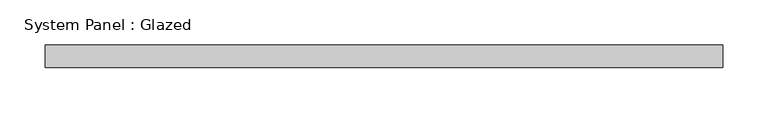
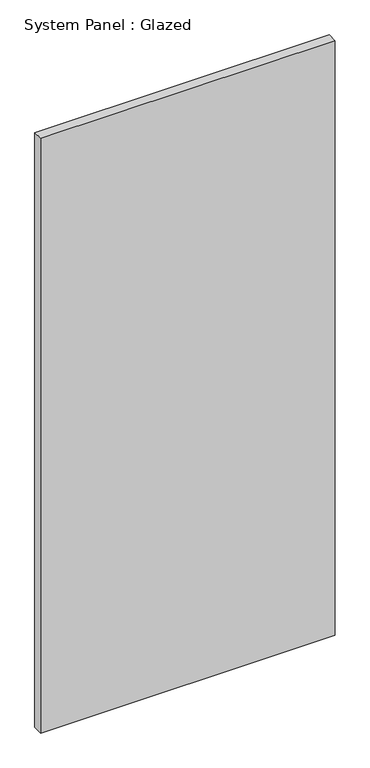
"""IFC4 building model written with IfcOpenShell, lengths in millimetres: plate geometry, System Panel : Glazed."""

from ifc_helpers import new_model, si_unit, origin, origin_with_axes, place, context, project, spatial, polyline, outline, extrude, source, transform, mapped, element, save


def system_panel_glazed_b6ba8a14(model_context):
    return source(origin(), model_context, "Body", "SweptSolid", [
        extrude(outline(polyline([(375.0, 24.5), (-375.0, 24.5), (-375.0, 49.5), (375.0, 49.5), (375.0, 24.5)])), origin_with_axes(), (0.0, 0.0, 1.0), 1600.0),
    ])


if __name__ == "__main__":
    model = new_model("IFC4")
    model_context = context("Model", 3, world=origin())
    ifc_project = project(units=[si_unit("LENGTHUNIT", "METRE", prefix="MILLI")], contexts=[model_context])
    site = spatial("IfcSite", under=ifc_project)
    building = spatial("IfcBuilding", under=site)
    placement = place(None, origin())
    system_panel_glazed_shape = system_panel_glazed_b6ba8a14(model_context)
    element("IfcPlate", 1, ObjectType="System Panel : Glazed", at=placement, inside=building, context=model_context, shape_type="MappedRepresentation", body=[
        mapped(system_panel_glazed_shape, transform((0.0, 0.0, 0.0), x_axis=(1.0, 0.0, 0.0), y_axis=(0.0, 1.0, 0.0), z_axis=(0.0, 0.0, 1.0))),
    ])
    save(model, "model.ifc")

# Revit data of these elements
# Type "System Panel : Glazed"
#   Construction Type Id = "GSP4R"
#   Analytic Construction = "1/8 in Pilkington single glazing"
#   Visual Light Transmittance = 0.9
#   Solar Heat Gain Coefficient = 0.86
#   Heat Transfer Coefficient (U) = 6.7069 W/(m²·K)
#   Define Thermal Properties by = 1
# Element 1 (IfcPlate, "System Panel : Glazed")
#   Materials on its faces: "Glass"
# Materials
#   "Glass": class "Glass", colour RGB 245 245 243, transparency 1, Description = "Soda Lime Glass", Cost = 0
